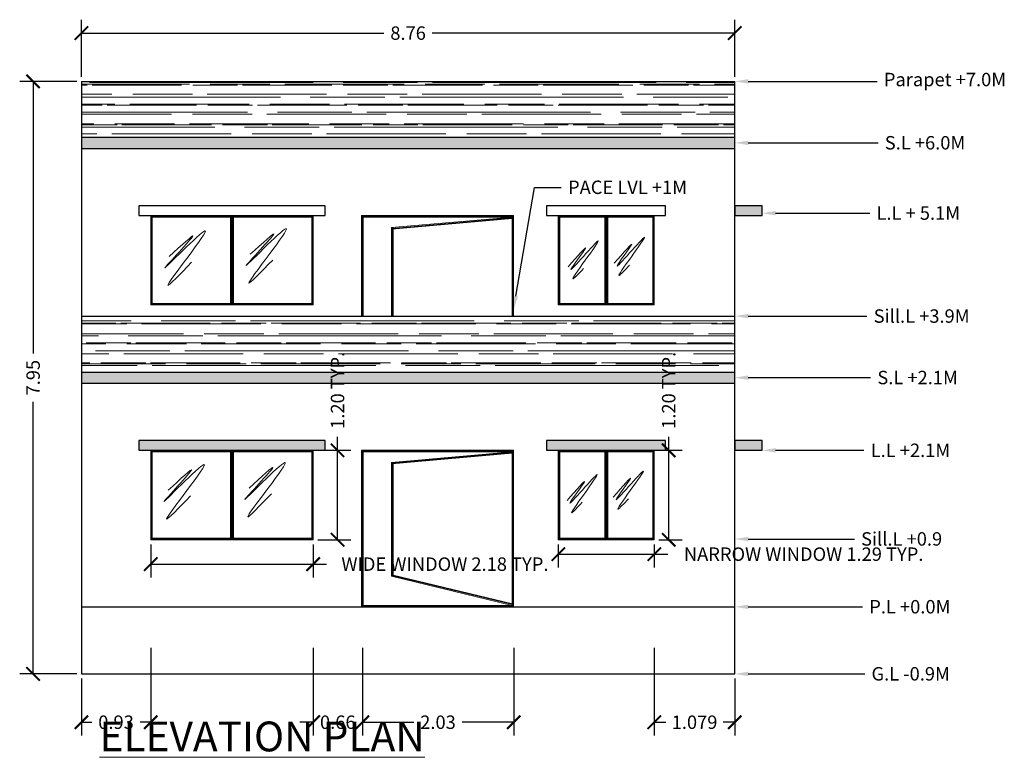
# Model space of a CAD drawing. Units: metres. Extents: x 6.8 to 74, y 0.6 to 37.
# Tile 2 of 5: x 6.8 to 20, y 19.5 to 29.4. Entities that reach past the tile are written whole.
import ezdxf
from ezdxf import colors
from ezdxf.entities.mleader import LeaderData, LeaderLine
from ezdxf.math import Vec2, Vec3

# ---------------------------------------------------------------- set-up
doc = ezdxf.new("R2010")
doc.units = ezdxf.units.M
doc.header["$LTSCALE"] = 0.2
doc.header["$MEASUREMENT"] = 0
for name, color, linetype, lineweight in [('A-ANNO-DIMS', 2, 'Continuous', 18), ('A-ANNO-SYMB', 3, 'Continuous', 18), ('A-ANNO-TEXT', 7, 'Continuous', 18), ('A-DOOR', 4, 'Continuous', 20), ('A-ELEV', 7, 'Continuous', 25), ('A-ELEV-PATT', 252, 'Continuous', 13), ('A-GLAZ', 4, 'Continuous', 18)]:
    doc.layers.add(name, color=color, linetype=linetype, lineweight=lineweight)
doc.styles.get("Standard").update_dxf_attribs({"font": 'arial.ttf'})
doc.dimstyles.get("Standard").update_dxf_attribs({"dimtxt": 0.18, "dimasz": 0.18, "dimexe": 0.18, "dimexo": 0.0625, "dimgap": 0.09, "dimtad": 0, "dimzin": 0, "dimdsep": 46, "dimtxsty": 'Standard', "dimblk": 'ARCHTICK', "dimcen": 0.09, "dimadec": 0, "dimazin": 0, "dimtfac": 1, "dimtofl": 0, "dimtmove": 0, "dimatfit": 3, "dimfxl": 1, "dimfxlon": 1, "dimtolj": 1, "dimtzin": 0, "dimarcsym": 0})

# ---------------------------------------------------------------- blocks, each defined once
blk = doc.blocks.new('WIN-ELEV-WIDE')
for p, q in [((1.069, 1.18), (1.069, 0.02)), ((1.079, 1.18), (1.079, 0.02)), ((1.089, 1.18), (1.089, 0.02)), ((1.099, 1.18), (1.099, 0.02)), ((1.109, 1.18), (1.109, 0.02))]:
    blk.add_line(p, q)
for points in [[(0, 1.2), (2.179, 1.2), (2.179, 0), (0, 0)], [(0.01, 1.19), (2.169, 1.19), (2.169, 0.01), (0.01, 0.01)], [(0.02, 1.18), (2.159, 1.18), (2.159, 0.02), (0.02, 0.02)]]:
    blk.add_lwpolyline(points, close=True)
blk = doc.blocks.new('WIN-ELEV-NARROW')
for p, q in [((0.623, 1.18), (0.623, 0.02)), ((0.633, 1.18), (0.633, 0.02)), ((0.643, 1.18), (0.643, 0.02)), ((0.653, 1.18), (0.653, 0.02)), ((0.663, 1.18), (0.663, 0.02))]:
    blk.add_line(p, q)
for points in [[(0, 1.2), (1.287, 1.2), (1.287, 0), (0, 0)], [(0.01, 1.19), (1.277, 1.19), (1.277, 0.01), (0.01, 0.01)], [(0.02, 1.18), (1.267, 1.18), (1.267, 0.02), (0.02, 0.02)]]:
    blk.add_lwpolyline(points, close=True)
blk = doc.blocks.new('GLASS-MARK-WIDE')
blk.add_open_spline([(0.474, 0.723), (0.638, 0.873), (1.025, 1.226), (0, 0.135), (1.505, 1.679), (0.148, 0), (0.617, 0.484), (0.774, 0.646)], degree=3, knots=[0, 0, 0, 0, 0.418458, 0.984648, 1.71487, 2.600392, 3.046341, 3.046341, 3.046341, 3.046341])
blk = doc.blocks.new('GLASS-MARK-NARROW')
blk.add_open_spline([(0.208, 0.362), (0.334, 0.505), (0.586, 0.792), (0, 0.016), (0.998, 1.186), (0.094, 0), (0.351, 0.272), (0.413, 0.338)], degree=3, knots=[0, 0, 0, 0, 0.340685, 0.684461, 1.213424, 1.827041, 2.025054, 2.025054, 2.025054, 2.025054])
blk = doc.blocks.new('_ArchTick')
at = {"color": 0, "linetype": 'ByBlock', "const_width": 0.15}
blk.add_lwpolyline([(-0.5, -0.5), (0.5, 0.5)], dxfattribs=at)
blk = doc.blocks.new('*D46')
at = {"layer": 'A-ANNO-DIMS', "color": 0, "lineweight": -2, "ltscale": 0.9, "transparency": 16777216}
for p, q in [((8.542, 22.402), (8.542, 21.957)), ((10.72, 22.402), (10.72, 21.957)), ((8.542, 22.137), (10.72, 22.137)), ((10.72, 22.137), (10.9, 22.137))]:
    blk.add_line(p, q, dxfattribs=at)
at = {"layer": 'Defpoints', "color": 0, "ltscale": 0.9, "transparency": 16777216}
for p in [(8.542, 22.464), (10.72, 22.464), (10.72, 22.137)]:
    blk.add_point(p, dxfattribs=at)
at = {"layer": 'A-ANNO-DIMS', "color": 0, "lineweight": -2, "ltscale": 0.9, "transparency": 16777216, "xscale": 0.18, "yscale": 0.18, "zscale": 0.18, "rotation": 180}
blk.add_blockref('_ArchTick', (8.542, 22.137), dxfattribs=at)
at = {"layer": 'A-ANNO-DIMS', "color": 0, "lineweight": -2, "ltscale": 0.9, "transparency": 16777216, "xscale": 0.18, "yscale": 0.18, "zscale": 0.18}
blk.add_blockref('_ArchTick', (10.72, 22.137), dxfattribs=at)
at = {"layer": 'A-ANNO-DIMS', "color": 0, "ltscale": 0.9, "transparency": 16777216, "insert": (12.487, 22.137), "char_height": 0.18, "attachment_point": 5}
blk.add_mtext('\\A1;WIDE WINDOW 2.18 TYP.', dxfattribs=at)
blk = doc.blocks.new('*D47')
at = {"layer": 'A-ANNO-DIMS', "color": 0, "lineweight": -2, "ltscale": 0.9, "transparency": 16777216}
for p, q in [((11.047, 23.664), (11.047, 23.844)), ((10.783, 23.664), (11.227, 23.664)), ((11.047, 22.464), (11.047, 23.664)), ((10.783, 22.464), (11.227, 22.464))]:
    blk.add_line(p, q, dxfattribs=at)
at = {"layer": 'Defpoints', "color": 0, "ltscale": 0.9, "transparency": 16777216}
for p in [(10.72, 23.664), (11.047, 23.664), (10.72, 22.464)]:
    blk.add_point(p, dxfattribs=at)
at = {"layer": 'A-ANNO-DIMS', "color": 0, "lineweight": -2, "ltscale": 0.9, "transparency": 16777216, "xscale": 0.18, "yscale": 0.18, "zscale": 0.18}
for p, rotation in [((11.047, 23.664), 90), ((11.047, 22.464), 270)]:
    blk.add_blockref('_ArchTick', p, dxfattribs=dict(at, rotation=rotation))
at = {"layer": 'A-ANNO-DIMS', "color": 0, "ltscale": 0.9, "transparency": 16777216, "insert": (11.047, 24.469), "char_height": 0.18, "attachment_point": 5, "rotation": 90}
blk.add_mtext('\\A1;1.20 TYP.', dxfattribs=at)
blk = doc.blocks.new('*D48')
at = {"layer": 'A-ANNO-DIMS', "color": 0, "lineweight": -2, "ltscale": 0.9, "transparency": 16777216}
for p, q in [((14.007, 22.402), (14.007, 22.091)), ((15.294, 22.402), (15.294, 22.091)), ((14.007, 22.271), (15.294, 22.271)), ((15.294, 22.271), (15.474, 22.271))]:
    blk.add_line(p, q, dxfattribs=at)
at = {"layer": 'Defpoints', "color": 0, "ltscale": 0.9, "transparency": 16777216}
for p in [(14.007, 22.464), (15.294, 22.464), (15.294, 22.271)]:
    blk.add_point(p, dxfattribs=at)
at = {"layer": 'A-ANNO-DIMS', "color": 0, "lineweight": -2, "ltscale": 0.9, "transparency": 16777216, "xscale": 0.18, "yscale": 0.18, "zscale": 0.18, "rotation": 180}
blk.add_blockref('_ArchTick', (14.007, 22.271), dxfattribs=at)
at = {"layer": 'A-ANNO-DIMS', "color": 0, "lineweight": -2, "ltscale": 0.9, "transparency": 16777216, "xscale": 0.18, "yscale": 0.18, "zscale": 0.18}
blk.add_blockref('_ArchTick', (15.294, 22.271), dxfattribs=at)
at = {"layer": 'A-ANNO-DIMS', "color": 0, "ltscale": 0.9, "transparency": 16777216, "insert": (17.297, 22.271), "char_height": 0.18, "attachment_point": 5}
blk.add_mtext('\\A1;NARROW WINDOW 1.29 TYP.', dxfattribs=at)
blk = doc.blocks.new('*D49')
at = {"layer": 'A-ANNO-DIMS', "color": 0, "lineweight": -2, "ltscale": 0.9, "transparency": 16777216}
for p, q in [((15.487, 23.664), (15.487, 23.844)), ((15.357, 23.664), (15.667, 23.664)), ((15.487, 22.464), (15.487, 23.664)), ((15.357, 22.464), (15.667, 22.464))]:
    blk.add_line(p, q, dxfattribs=at)
at = {"layer": 'Defpoints', "color": 0, "ltscale": 0.9, "transparency": 16777216}
for p in [(15.294, 23.664), (15.487, 23.664), (15.294, 22.464)]:
    blk.add_point(p, dxfattribs=at)
at = {"layer": 'A-ANNO-DIMS', "color": 0, "lineweight": -2, "ltscale": 0.9, "transparency": 16777216, "xscale": 0.18, "yscale": 0.18, "zscale": 0.18}
for p, rotation in [((15.487, 23.664), 90), ((15.487, 22.464), 270)]:
    blk.add_blockref('_ArchTick', p, dxfattribs=dict(at, rotation=rotation))
at = {"layer": 'A-ANNO-DIMS', "color": 0, "ltscale": 0.9, "transparency": 16777216, "insert": (15.487, 24.469), "char_height": 0.18, "attachment_point": 5, "rotation": 90}
blk.add_mtext('\\A1;1.20 TYP.', dxfattribs=at)
blk = doc.blocks.new('*D50')
at = {"layer": 'A-ANNO-DIMS', "color": 0, "lineweight": -2, "ltscale": 0.9, "transparency": 16777216}
for p, q in [((7.613, 28.677), (7.613, 29.442)), ((16.373, 28.677), (16.373, 29.442)), ((7.613, 29.262), (11.669, 29.262)), ((16.373, 29.262), (12.317, 29.262))]:
    blk.add_line(p, q, dxfattribs=at)
at = {"layer": 'Defpoints', "color": 0, "ltscale": 0.9, "transparency": 16777216}
for p in [(16.373, 29.262), (7.613, 28.614), (16.373, 28.614)]:
    blk.add_point(p, dxfattribs=at)
at = {"layer": 'A-ANNO-DIMS', "color": 0, "lineweight": -2, "ltscale": 0.9, "transparency": 16777216, "xscale": 0.18, "yscale": 0.18, "zscale": 0.18, "rotation": 180}
blk.add_blockref('_ArchTick', (7.613, 29.262), dxfattribs=at)
at = {"layer": 'A-ANNO-DIMS', "color": 0, "lineweight": -2, "ltscale": 0.9, "transparency": 16777216, "xscale": 0.18, "yscale": 0.18, "zscale": 0.18}
blk.add_blockref('_ArchTick', (16.373, 29.262), dxfattribs=at)
at = {"layer": 'A-ANNO-DIMS', "color": 0, "ltscale": 0.9, "transparency": 16777216, "insert": (11.993, 29.262), "char_height": 0.18, "attachment_point": 5}
blk.add_mtext('\\A1;8.76', dxfattribs=at)
blk = doc.blocks.new('*D51')
at = {"layer": 'A-ANNO-DIMS', "color": 0, "lineweight": -2, "ltscale": 0.9, "transparency": 16777216}
for p, q in [((7.551, 28.614), (6.785, 28.614)), ((6.965, 28.614), (6.965, 24.963)), ((6.965, 20.664), (6.965, 24.315)), ((7.551, 20.664), (6.785, 20.664))]:
    blk.add_line(p, q, dxfattribs=at)
at = {"layer": 'Defpoints', "color": 0, "ltscale": 0.9, "transparency": 16777216}
for p in [(6.965, 28.614), (7.613, 28.614), (7.613, 20.664)]:
    blk.add_point(p, dxfattribs=at)
at = {"layer": 'A-ANNO-DIMS', "color": 0, "lineweight": -2, "ltscale": 0.9, "transparency": 16777216, "xscale": 0.18, "yscale": 0.18, "zscale": 0.18}
for p, rotation in [((6.965, 28.614), 90), ((6.965, 20.664), 270)]:
    blk.add_blockref('_ArchTick', p, dxfattribs=dict(at, rotation=rotation))
at = {"layer": 'A-ANNO-DIMS', "color": 0, "ltscale": 0.9, "transparency": 16777216, "insert": (6.965, 24.639), "char_height": 0.18, "attachment_point": 5, "rotation": 90}
blk.add_mtext('\\A1;7.95', dxfattribs=at)
blk = doc.blocks.new('*D52')
at = {"layer": 'A-ANNO-DIMS', "color": 0, "lineweight": -2, "ltscale": 0.9, "transparency": 16777216}
for p, q in [((8.542, 21.016), (8.542, 19.836)), ((7.613, 20.602), (7.613, 19.836)), ((7.613, 20.016), (7.754, 20.016)), ((8.542, 20.016), (8.401, 20.016))]:
    blk.add_line(p, q, dxfattribs=at)
at = {"layer": 'Defpoints', "color": 0, "ltscale": 0.9, "transparency": 16777216}
for p in [(8.542, 22.464), (7.613, 20.664), (8.542, 20.016)]:
    blk.add_point(p, dxfattribs=at)
at = {"layer": 'A-ANNO-DIMS', "color": 0, "lineweight": -2, "ltscale": 0.9, "transparency": 16777216, "xscale": 0.18, "yscale": 0.18, "zscale": 0.18, "rotation": 180}
blk.add_blockref('_ArchTick', (7.613, 20.016), dxfattribs=at)
at = {"layer": 'A-ANNO-DIMS', "color": 0, "lineweight": -2, "ltscale": 0.9, "transparency": 16777216, "xscale": 0.18, "yscale": 0.18, "zscale": 0.18}
blk.add_blockref('_ArchTick', (8.542, 20.016), dxfattribs=at)
at = {"layer": 'A-ANNO-DIMS', "color": 0, "ltscale": 0.9, "transparency": 16777216, "insert": (8.077, 20.016), "char_height": 0.18, "attachment_point": 5}
blk.add_mtext('\\A1;0.93', dxfattribs=at)
blk = doc.blocks.new('*D53')
at = {"layer": 'A-ANNO-DIMS', "color": 0, "lineweight": -2, "ltscale": 0.9, "transparency": 16777216}
for p, q in [((10.720259, 21.016051), (10.720259, 19.836051)), ((11.380027, 21.016051), (11.380027, 19.836051)), ((10.720259, 20.016051), (10.540259, 20.016051)), ((11.380027, 20.016051), (11.560027, 20.016051))]:
    blk.add_line(p, q, dxfattribs=at)
at = {"layer": 'Defpoints', "color": 0, "ltscale": 0.9, "transparency": 16777216}
for p in [(10.720259, 22.464051), (11.380027, 21.574051), (11.380027, 20.016051)]:
    blk.add_point(p, dxfattribs=at)
at = {"layer": 'A-ANNO-DIMS', "color": 0, "lineweight": -2, "ltscale": 0.9, "transparency": 16777216, "xscale": 0.18, "yscale": 0.18, "zscale": 0.18}
blk.add_blockref('_ArchTick', (10.720259, 20.016051), dxfattribs=at)
at = {"layer": 'A-ANNO-DIMS', "color": 0, "lineweight": -2, "ltscale": 0.9, "transparency": 16777216, "xscale": 0.18, "yscale": 0.18, "zscale": 0.18, "rotation": 180}
blk.add_blockref('_ArchTick', (11.380027, 20.016051), dxfattribs=at)
at = {"layer": 'A-ANNO-DIMS', "color": 0, "ltscale": 0.9, "transparency": 16777216, "insert": (11.050143, 20.016051), "char_height": 0.18, "attachment_point": 5}
blk.add_mtext('\\A1;0.66', dxfattribs=at)
blk = doc.blocks.new('*D54')
at = {"layer": 'A-ANNO-DIMS', "color": 0, "lineweight": -2, "ltscale": 0.9, "transparency": 16777216}
for p, q in [((11.38, 21.016), (11.38, 19.836)), ((13.409, 21.016), (13.409, 19.836)), ((11.38, 20.016), (12.069, 20.016)), ((13.409, 20.016), (12.72, 20.016))]:
    blk.add_line(p, q, dxfattribs=at)
at = {"layer": 'Defpoints', "color": 0, "ltscale": 0.9, "transparency": 16777216}
for p in [(11.38, 21.574), (13.409, 21.564), (13.409, 20.016)]:
    blk.add_point(p, dxfattribs=at)
at = {"layer": 'A-ANNO-DIMS', "color": 0, "lineweight": -2, "ltscale": 0.9, "transparency": 16777216, "xscale": 0.18, "yscale": 0.18, "zscale": 0.18, "rotation": 180}
blk.add_blockref('_ArchTick', (11.38, 20.016), dxfattribs=at)
at = {"layer": 'A-ANNO-DIMS', "color": 0, "lineweight": -2, "ltscale": 0.9, "transparency": 16777216, "xscale": 0.18, "yscale": 0.18, "zscale": 0.18}
blk.add_blockref('_ArchTick', (13.409, 20.016), dxfattribs=at)
at = {"layer": 'A-ANNO-DIMS', "color": 0, "ltscale": 0.9, "transparency": 16777216, "insert": (12.394, 20.016), "char_height": 0.18, "attachment_point": 5}
blk.add_mtext('\\A1;2.03', dxfattribs=at)
blk = doc.blocks.new('*D55')
at = {"layer": 'A-ANNO-DIMS', "color": 0, "lineweight": -2, "ltscale": 0.9, "transparency": 16777216}
for p, q in [((15.294, 21.016), (15.294, 19.836)), ((16.373, 20.602), (16.373, 19.836)), ((15.294, 20.016), (15.448, 20.016)), ((16.373, 20.016), (16.219, 20.016))]:
    blk.add_line(p, q, dxfattribs=at)
at = {"layer": 'Defpoints', "color": 0, "ltscale": 0.9, "transparency": 16777216}
for p in [(15.294, 22.464), (16.373, 20.664), (16.373, 20.016)]:
    blk.add_point(p, dxfattribs=at)
at = {"layer": 'A-ANNO-DIMS', "color": 0, "lineweight": -2, "ltscale": 0.9, "transparency": 16777216, "xscale": 0.18, "yscale": 0.18, "zscale": 0.18, "rotation": 180}
blk.add_blockref('_ArchTick', (15.294, 20.016), dxfattribs=at)
at = {"layer": 'A-ANNO-DIMS', "color": 0, "lineweight": -2, "ltscale": 0.9, "transparency": 16777216, "xscale": 0.18, "yscale": 0.18, "zscale": 0.18}
blk.add_blockref('_ArchTick', (16.373, 20.016), dxfattribs=at)
at = {"layer": 'A-ANNO-DIMS', "color": 0, "ltscale": 0.9, "transparency": 16777216, "insert": (15.834, 20.016), "char_height": 0.18, "attachment_point": 5}
blk.add_mtext('\\A1;1.079', dxfattribs=at)

msp = doc.modelspace()

# ---------------------------------------------------------------- hatches: boundary and pattern name
at = {"layer": 'A-ELEV-PATT'}
h = msp.add_hatch(dxfattribs=at)
h.set_pattern_fill('AR-RROOF', color=256, scale=0.2)
h.paths.add_polyline_path([(16.3731, 28.6141), (7.6131, 28.6141), (7.6131, 27.8641), (16.3731, 27.8641)])
h.paths.add_polyline_path([(16.3731, 25.4641), (7.6131, 25.4641), (7.6131, 24.7141), (16.3731, 24.7141)])
h = msp.add_hatch(color=256, dxfattribs=at)
h.dxf.hatch_style = 1
h.paths.add_polyline_path([(16.3731, 24.7141), (7.6131, 24.7141), (7.6131, 24.5641), (16.3731, 24.5641)])
h.paths.add_polyline_path([(16.3731, 27.8641), (7.6131, 27.8641), (7.6131, 27.7141), (16.3731, 27.7141)])
h.paths.add_polyline_path([(10.879, 23.7952), (8.3816, 23.7952), (8.3816, 23.6641), (10.879, 23.6641)])
h.paths.add_polyline_path([(15.4454, 23.7952), (13.8494, 23.7952), (13.8494, 23.6641), (15.4454, 23.6641)])
h = msp.add_hatch(color=256, dxfattribs=at)
h.dxf.hatch_style = 1
h.paths.add_polyline_path([(16.7402, 23.7952), (16.3731, 23.7952), (16.3731, 23.6641), (16.7402, 23.6641)])
h.paths.add_polyline_path([(16.7402, 26.9452), (16.3731, 26.9452), (16.3731, 26.8141), (16.7402, 26.8141)])

# ---------------------------------------------------------------- linework, layer by layer
at = {"layer": 'A-DOOR'}
for p, q in [((11.7713, 26.6518), (13.3885, 26.7941)), ((11.7721, 26.6419), (13.3894, 26.7841)), ((11.773, 26.6319), (13.3903, 26.7741)), ((11.7713, 26.6518), (11.7713, 25.4641)), ((11.7813, 26.6518), (11.7813, 25.4641)), ((11.7913, 26.6518), (11.7913, 25.4641)), ((11.7713, 23.5018), (13.3885, 23.6441)), ((11.7721, 23.4919), (13.3894, 23.6341)), ((11.7713, 23.5018), (11.7713, 21.975)), ((11.773, 23.4819), (13.3903, 23.6241)), ((11.7813, 23.5018), (11.7813, 21.975)), ((11.7913, 23.5018), (11.7913, 21.975)), ((11.7713, 21.975), (13.3885, 21.5841)), ((11.7736, 21.9848), (13.3909, 21.5938)), ((11.776, 21.9945), (13.3932, 21.6035))]:
    msp.add_line(p, q, dxfattribs=at)
for points in [[(11.37, 25.4641), (11.37, 26.8141), (13.4085, 26.8141), (13.4085, 25.4641)], [(11.38, 25.4641), (11.38, 26.8041), (13.3985, 26.8041), (13.3985, 25.4641)], [(11.39, 25.4641), (11.39, 26.7941), (13.3885, 26.7941), (13.3885, 25.4641)], [(13.4085, 24.7141), (11.37, 24.7141)]]:
    msp.add_lwpolyline(points, dxfattribs=at)
for points in [[(11.37, 23.6641), (13.4085, 23.6641), (13.4085, 21.5641), (11.37, 21.5641)], [(11.38, 23.6541), (13.3985, 23.6541), (13.3985, 21.5741), (11.38, 21.5741)], [(11.39, 23.6441), (13.3885, 23.6441), (13.3885, 21.5841), (11.39, 21.5841)]]:
    msp.add_lwpolyline(points, close=True, dxfattribs=at)
at = {"layer": 'A-ELEV'}
for p, q in [((7.6131, 28.6141), (16.3731, 28.6141)), ((7.6131, 28.6141), (7.6131, 27.8641)), ((16.3731, 27.8641), (16.3731, 28.6141)), ((7.6131, 27.8641), (16.3731, 27.8641)), ((7.6131, 27.8641), (7.6131, 27.7141)), ((16.3731, 27.7141), (16.3731, 27.8641)), ((7.6131, 27.7141), (16.3731, 27.7141)), ((7.6131, 27.7141), (7.6131, 24.7141)), ((16.3731, 24.7141), (16.3731, 27.7141)), ((7.6131, 25.4641), (16.3731, 25.4641)), ((7.6131, 25.4641), (7.6131, 24.7141)), ((16.3731, 24.7141), (16.3731, 25.4641)), ((7.6131, 24.7141), (16.3731, 24.7141)), ((7.6131, 24.7141), (7.6131, 24.5641)), ((16.3731, 24.5641), (16.3731, 24.7141)), ((7.6131, 24.5641), (16.3731, 24.5641)), ((7.6131, 24.5641), (7.6131, 21.5641)), ((16.3731, 21.5641), (16.3731, 24.5641)), ((7.6131, 21.5641), (16.3731, 21.5641)), ((7.6131, 21.5641), (7.6131, 20.6641)), ((16.3731, 20.6641), (16.3731, 21.5641)), ((7.6131, 20.6641), (16.3731, 20.6641))]:
    msp.add_line(p, q, dxfattribs=at)
for points in [[(8.3816, 26.8141), (10.879, 26.8141), (10.879, 26.9452), (8.3816, 26.9452)], [(13.8494, 26.8141), (15.4454, 26.8141), (15.4454, 26.9452), (13.8494, 26.9452)], [(16.3731, 26.8141), (16.7402, 26.8141), (16.7402, 26.9452), (16.3731, 26.9452)], [(8.3816, 23.6641), (10.879, 23.6641), (10.879, 23.7952), (8.3816, 23.7952)], [(13.8494, 23.6641), (15.4454, 23.6641), (15.4454, 23.7952), (13.8494, 23.7952)], [(16.3731, 23.6641), (16.7402, 23.6641), (16.7402, 23.7952), (16.3731, 23.7952)]]:
    msp.add_lwpolyline(points, close=True, dxfattribs=at)

# ---------------------------------------------------------------- block references
at = {"layer": 'A-GLAZ'}
for name, p in [('WIN-ELEV-WIDE', (8.5416, 25.6141)), ('WIN-ELEV-NARROW', (14.0073, 25.6141)), ('GLASS-MARK-WIDE', (8.3166, 25.5421)), ('GLASS-MARK-WIDE', (9.4033, 25.5714)), ('GLASS-MARK-NARROW', (13.931, 25.7653)), ('GLASS-MARK-NARROW', (14.55, 25.8119)), ('WIN-ELEV-WIDE', (8.5416, 22.4641)), ('WIN-ELEV-NARROW', (14.0073, 22.4641)), ('GLASS-MARK-WIDE', (9.3885, 22.4352)), ('GLASS-MARK-WIDE', (8.3018, 22.4059)), ('GLASS-MARK-NARROW', (14.5352, 22.6757)), ('GLASS-MARK-NARROW', (13.9161, 22.6292))]:
    msp.add_blockref(name, p, dxfattribs=at)

# ---------------------------------------------------------------- texts
at = {"layer": 'A-ANNO-TEXT', "insert": (7.8549, 20.0251), "char_height": 0.4, "attachment_point": 1}
msp.add_mtext_dynamic_manual_height_columns('{\\LELEVATION PLAN}', width=7.004508, gutter_width=1, heights=[0], dxfattribs=at)

# ---------------------------------------------------------------- dimensions: what is measured, and where the dimension line sits
at = {"layer": 'A-ANNO-DIMS', "ltscale": 0.9}
for base, p1, p2, override, picture, middle in [((16.3731, 29.2621), (7.6131, 28.6141), (16.3731, 28.6141), {"dimdec": 2, "dimlfac": 1, "dimrnd": 0, "dimzin": 0, "dimdsep": 46, "dimlunit": 2}, '*D50', (11.9931, 29.2621)), ((8.5416, 20.0161), (7.6131, 20.6641), (8.5416, 22.4641), {"dimdec": 2, "dimlfac": 1, "dimrnd": 0, "dimzin": 0, "dimdsep": 46, "dimlunit": 2}, '*D52', (8.0773, 20.0161)), ((11.38, 20.0161), (10.7203, 22.4641), (11.38, 21.5741), {"dimdec": 2, "dimlfac": 1, "dimrnd": 0, "dimzin": 0, "dimdsep": 46, "dimlunit": 2}, '*D53', (11.0501, 20.0161)), ((16.3731, 20.0161), (15.2941, 22.4641), (16.3731, 20.6641), {"dimdec": 3, "dimlfac": 1, "dimrnd": 0, "dimzin": 0, "dimdsep": 46, "dimlunit": 2}, '*D55', (15.8336, 20.0161)), ((13.4085, 20.0161), (11.38, 21.5741), (13.4085, 21.5641), {"dimdec": 2, "dimlfac": 1, "dimrnd": 0, "dimzin": 0, "dimdsep": 46, "dimlunit": 2}, '*D54', (12.3943, 20.0161))]:
    dim = msp.add_linear_dim(base=base, p1=p1, p2=p2, dimstyle='Standard', override=override, dxfattribs=at)
    dim.commit()
    dim.dimension.update_dxf_attribs({"geometry": picture, "text_midpoint": middle})
dim = msp.add_linear_dim(base=(6.9651, 28.6141), p1=(7.6131, 20.6641), p2=(7.6131, 28.6141), angle=90, dimstyle='Standard', override={"dimdec": 2, "dimlfac": 1, "dimrnd": 0, "dimzin": 0, "dimdsep": 46, "dimlunit": 2}, dxfattribs=at)
dim.commit()
dim.dimension.update_dxf_attribs({"geometry": '*D51', "text_midpoint": (6.9651, 24.6391)})
for base, p1, p2, picture, middle in [((11.0471, 23.6641), (10.7203, 22.4641), (10.7203, 23.6641), '*D47', (11.0471, 24.4685)), ((15.4871, 23.6641), (15.2941, 22.4641), (15.2941, 23.6641), '*D49', (15.4871, 24.4685))]:
    dim = msp.add_linear_dim(base=base, p1=p1, p2=p2, angle=90, text='<> TYP.', dimstyle='Standard', override={"dimdec": 2, "dimlfac": 1, "dimrnd": 0, "dimzin": 0, "dimdsep": 46, "dimlunit": 2}, dxfattribs=at)
    dim.commit()
    dim.dimension.update_dxf_attribs({"geometry": picture, "text_midpoint": middle})
for base, p1, p2, text, picture, middle in [((15.2941, 22.271), (14.0073, 22.4641), (15.2941, 22.4641), 'NARROW WINDOW <> TYP.', '*D48', (17.297, 22.271)), ((10.7203, 22.1373), (8.5416, 22.4641), (10.7203, 22.4641), 'WIDE WINDOW <> TYP.', '*D46', (12.4867, 22.1373))]:
    dim = msp.add_linear_dim(base=base, p1=p1, p2=p2, text=text, dimstyle='Standard', override={"dimdec": 2, "dimlfac": 1, "dimrnd": 0, "dimzin": 0, "dimdsep": 46, "dimlunit": 2}, dxfattribs=at)
    dim.commit()
    dim.dimension.update_dxf_attribs({"geometry": picture, "text_midpoint": middle})

# ---------------------------------------------------------------- leaders
at = {"layer": 'A-ANNO-SYMB'}
ml = msp.add_multileader_mtext('Standard', dxfattribs=at)
ml.set_content('Parapet +7.0M', color=256)
ml.set_leader_properties()
ml.build(insert=Vec2(0, 0))
ml.multileader.update_dxf_attribs({"dogleg_length": 0.36, "arrow_head_size": 0.18})
ctx = ml.context
ctx.base_point, ctx.char_height, ctx.arrow_head_size, ctx.landing_gap_size, ctx.plane_origin = Vec3(18.2825, 28.6141), 0.18, 0.18, 0.09, Vec3(16.3731, 28.6141)
notes = []
notes.append((ctx, [(0, (1, 1, 0), (17.9225, 28.6141), (1, 0), 0.36, [(0, [(16.3731, 28.6141)], 0, [])])]))
ctx.mtext.insert, ctx.mtext.flow_direction = Vec3(18.3725, 28.729), 5
ml = msp.add_multileader_mtext('Standard', dxfattribs=at)
ml.set_content('S.L +6.0M', color=256)
ml.set_leader_properties()
ml.build(insert=Vec2(0, 0))
ml.multileader.update_dxf_attribs({"dogleg_length": 0.36, "arrow_head_size": 0.18})
ctx = ml.context
ctx.base_point, ctx.char_height, ctx.arrow_head_size, ctx.landing_gap_size, ctx.plane_origin = Vec3(18.2949, 27.7891), 0.18, 0.18, 0.09, Vec3(16.3731, 27.7891)
notes.append((ctx, [(0, (1, 1, 0), (17.9349, 27.7891), (1, 0), 0.36, [(0, [(16.3731, 27.7891)], 0, [])])]))
ctx.mtext.insert, ctx.mtext.flow_direction = Vec3(18.3849, 27.8806), 5
ml = msp.add_multileader_mtext('Standard', dxfattribs=at)
ml.set_content('PACE LVL +1M', color=256)
ml.set_leader_properties()
ml.build(insert=Vec2(0, 0))
ml.multileader.update_dxf_attribs({"dogleg_length": 0.36, "arrow_head_size": 0.18})
ctx = ml.context
ctx.base_point, ctx.char_height, ctx.arrow_head_size, ctx.landing_gap_size, ctx.plane_origin = Vec3(14.0473, 27.1918), 0.18, 0.18, 0.09, Vec3(13.4085, 25.5554)
notes.append((ctx, [(0, (1, 1, 0), (13.6873, 27.1918), (1, 0), 0.36, [(0, [(13.4085, 25.5554)], 0, [])])]))
ctx.mtext.insert, ctx.mtext.flow_direction = Vec3(14.1373, 27.2833), 5
ml = msp.add_multileader_mtext('Standard', dxfattribs=at)
ml.set_content('L.L + 5.1M', color=256)
ml.set_leader_properties()
ml.build(insert=Vec2(0, 0))
ml.multileader.update_dxf_attribs({"dogleg_length": 0.36, "arrow_head_size": 0.18})
ctx = ml.context
ctx.base_point, ctx.char_height, ctx.arrow_head_size, ctx.landing_gap_size, ctx.plane_origin = Vec3(18.1834, 26.8457), 0.18, 0.18, 0.09, Vec3(16.7402, 26.8457)
notes.append((ctx, [(0, (1, 1, 0), (17.8234, 26.8457), (1, 0), 0.36, [(0, [(16.7402, 26.8457)], 0, [])])]))
ctx.mtext.insert, ctx.mtext.flow_direction = Vec3(18.2734, 26.9373), 5
ml = msp.add_multileader_mtext('Standard', dxfattribs=at)
ml.set_content('Sill.L +3.9M', color=256)
ml.set_leader_properties()
ml.build(insert=Vec2(0, 0))
ml.multileader.update_dxf_attribs({"dogleg_length": 0.36, "arrow_head_size": 0.18})
ctx = ml.context
ctx.base_point, ctx.char_height, ctx.arrow_head_size, ctx.landing_gap_size, ctx.plane_origin = Vec3(18.1456, 25.4641), 0.18, 0.18, 0.09, Vec3(16.3731, 25.4641)
notes.append((ctx, [(0, (1, 1, 0), (17.7856, 25.4641), (1, 0), 0.36, [(0, [(16.3731, 25.4641)], 0, [])])]))
ctx.mtext.insert, ctx.mtext.flow_direction = Vec3(18.2356, 25.5556), 5
ml = msp.add_multileader_mtext('Standard', dxfattribs=at)
ml.set_content('S.L +2.1M', color=256)
ml.set_leader_properties()
ml.build(insert=Vec2(0, 0))
ml.multileader.update_dxf_attribs({"dogleg_length": 0.36, "arrow_head_size": 0.18})
ctx = ml.context
ctx.base_point, ctx.char_height, ctx.arrow_head_size, ctx.landing_gap_size, ctx.plane_origin = Vec3(18.1952, 24.6391), 0.18, 0.18, 0.09, Vec3(16.3731, 24.6391)
notes.append((ctx, [(0, (1, 1, 0), (17.8352, 24.6391), (1, 0), 0.36, [(0, [(16.3731, 24.6391)], 0, [])])]))
ctx.mtext.insert, ctx.mtext.flow_direction = Vec3(18.2852, 24.7306), 5
ml = msp.add_multileader_mtext('Standard', dxfattribs=at)
ml.set_content('L.L +2.1M', color=256)
ml.set_leader_properties()
ml.build(insert=Vec2(0, 0))
ml.multileader.update_dxf_attribs({"dogleg_length": 0.36, "arrow_head_size": 0.18})
ctx = ml.context
ctx.base_point, ctx.char_height, ctx.arrow_head_size, ctx.landing_gap_size, ctx.plane_origin = Vec3(18.106, 23.6641), 0.18, 0.18, 0.09, Vec3(16.7402, 23.6641)
notes.append((ctx, [(0, (1, 1, 0), (17.746, 23.6641), (1, 0), 0.36, [(0, [(16.7402, 23.6641)], 0, [])])]))
ctx.mtext.insert, ctx.mtext.flow_direction = Vec3(18.196, 23.7541), 5
ml = msp.add_multileader_mtext('Standard', dxfattribs=at)
ml.set_content('Sill.L +0.9', color=256)
ml.set_leader_properties()
ml.build(insert=Vec2(0, 0))
ml.multileader.update_dxf_attribs({"dogleg_length": 0.36, "arrow_head_size": 0.18})
ctx = ml.context
ctx.base_point, ctx.char_height, ctx.arrow_head_size, ctx.landing_gap_size, ctx.plane_origin = Vec3(17.9771, 22.4739), 0.18, 0.18, 0.09, Vec3(16.3731, 22.4739)
notes.append((ctx, [(0, (1, 1, 0), (17.6171, 22.4739), (1, 0), 0.36, [(0, [(16.3731, 22.4739)], 0, [])])]))
ctx.mtext.insert, ctx.mtext.flow_direction = Vec3(18.0671, 22.5654), 5
ml = msp.add_multileader_mtext('Standard', dxfattribs=at)
ml.set_content('P.L +0.0M', color=256)
ml.set_leader_properties()
ml.build(insert=Vec2(0, 0))
ml.multileader.update_dxf_attribs({"dogleg_length": 0.36, "arrow_head_size": 0.18})
ctx = ml.context
ctx.base_point, ctx.char_height, ctx.arrow_head_size, ctx.landing_gap_size, ctx.plane_origin = Vec3(18.0864, 21.5641), 0.18, 0.18, 0.09, Vec3(16.3731, 21.5641)
notes.append((ctx, [(0, (1, 1, 0), (17.7264, 21.5641), (1, 0), 0.36, [(0, [(16.3731, 21.5641)], 0, [])])]))
ctx.mtext.insert, ctx.mtext.flow_direction = Vec3(18.1764, 21.6556), 5
ml = msp.add_multileader_mtext('Standard', dxfattribs=at)
ml.set_content('G.L -0.9M', color=256)
ml.set_leader_properties()
ml.build(insert=Vec2(0, 0))
ml.multileader.update_dxf_attribs({"dogleg_length": 0.36, "arrow_head_size": 0.18})
ctx = ml.context
ctx.base_point, ctx.char_height, ctx.arrow_head_size, ctx.landing_gap_size, ctx.plane_origin = Vec3(18.1163, 20.6641), 0.18, 0.18, 0.09, Vec3(16.3731, 20.6641)
notes.append((ctx, [(0, (1, 1, 0), (17.7563, 20.6641), (1, 0), 0.36, [(0, [(16.3731, 20.6641)], 0, [])])]))
ctx.mtext.insert, ctx.mtext.flow_direction = Vec3(18.2063, 20.7556), 5
for ctx, leaders in notes:
    for number, flags, end, landing, length, lines in leaders:
        leader = LeaderData()
        leader.index, (leader.has_last_leader_line, leader.has_dogleg_vector, leader.attachment_direction) = number, flags
        leader.last_leader_point, leader.dogleg_vector, leader.dogleg_length = Vec3(end), Vec3(landing), length
        for number, points, colour, breaks in lines:
            line = LeaderLine()
            line.index, line.vertices, line.color, line.breaks = number, Vec3.list(points), colors.encode_raw_color(colour), breaks
            leader.lines.append(line)
        ctx.leaders.append(leader)

doc.saveas('drawing.dxf')
